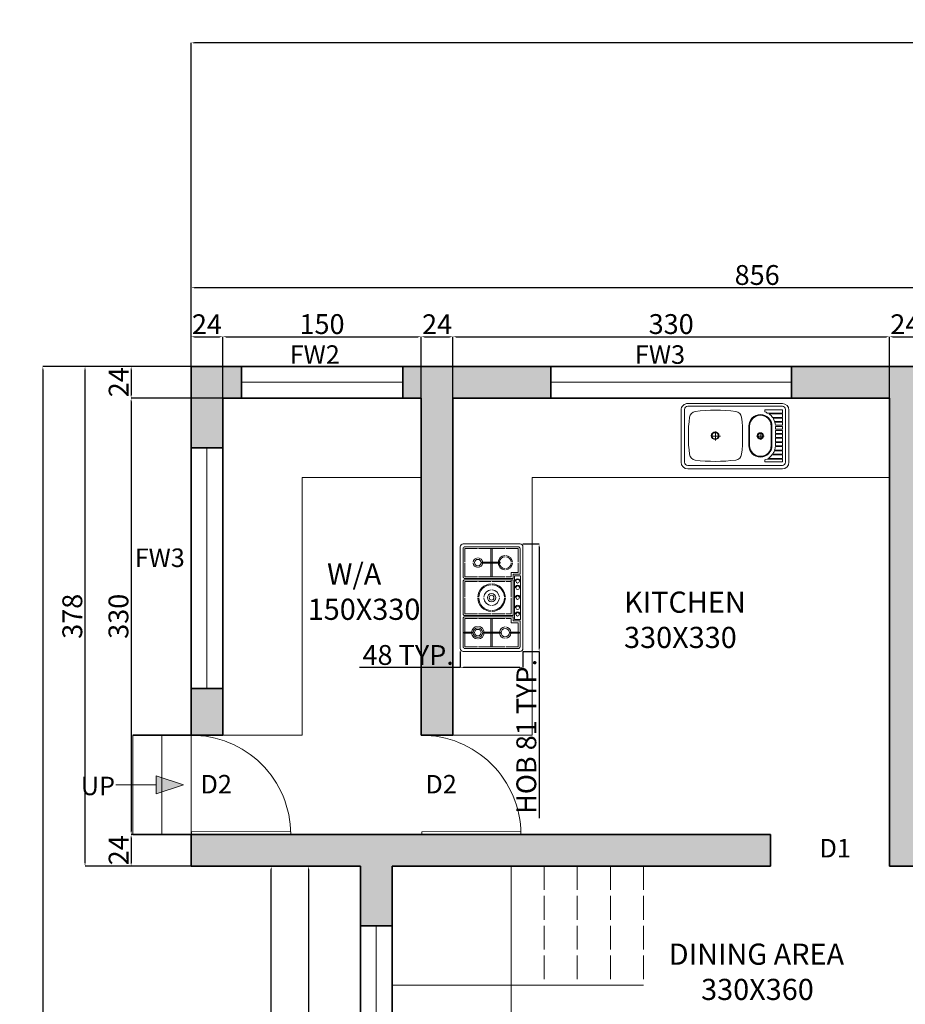
# Model space of a CAD drawing. Units: centimetres. Extents: x 2449 to 7478, y 778 to 2486.
# Tile 3 of 9: x 2449 to 3118, y 1732 to 2477. Entities that reach past the tile are written whole.
import ezdxf

# ---------------------------------------------------------------- set-up
doc = ezdxf.new("R2010")
doc.units = ezdxf.units.CM
doc.linetypes.add('ACAD_ISO02W100', pattern=[15, 12, -3])
for name, color, linetype, lineweight in [('A-ANNO-DIMS', 2, 'Continuous', 18), ('A-ANNO-SYMB', 8, 'Continuous', 18), ('A-ANNO-TEXT', 7, 'Continuous', 18), ('A-AREA-IDEN', 7, 'Continuous', 18), ('A-DOOR', 4, 'Continuous', 18), ('A-EQPM', 8, 'Continuous', 18), ('A-FLOR-CASE', 8, 'Continuous', 18), ('A-FLOR-FIXT', 8, 'Continuous', 18), ('A-FLOR-STRS', 7, 'Continuous', 18), ('A-FLOR-STRS-OVHD', 7, 'ACAD_ISO02W100', 13), ('A-WALL', 7, 'Continuous', 35), ('A-WALL-PATT', 7, 'Continuous', 13), ('Win', 1, 'Continuous', 18)]:
    doc.layers.add(name, color=color, linetype=linetype, lineweight=lineweight)
doc.styles.get("Standard").update_dxf_attribs({"font": 'arial.ttf'})
doc.dimstyles.new('ISO-25', dxfattribs={"dimtxt": 15, "dimasz": 2.5, "dimexe": 0, "dimexo": 0, "dimgap": 0, "dimtad": 1, "dimtxsty": 'Standard', "dimcen": 2.5, "dimadec": 0, "dimazin": 0, "dimtfac": 1, "dimtmove": 0, "dimatfit": 3, "dimfxl": 1, "dimarcsym": 0})

# ---------------------------------------------------------------- blocks, each defined once
blk = doc.blocks.new('sink 1')
for points in [[(-7.34, 1.48), (-7.34, 22.73)], [(-6.56, 1.48), (-6.56, 22.73)], [(5.86, 24.22), (-5.86, 24.22)], [(6.01, 23.43), (-5.86, 23.43)], [(6.72, 1.48), (6.72, 22.73)], [(7.34, 1.48), (7.34, 22.73)], [(1.09, 16.48), (-0.94, 16.48)], [(0, 15.39), (0, 17.42)], [(-2.09, 8.99), (2.28, 8.99)], [(-2.09, 8.84), (2.28, 8.84)], [(0, 5.55), (0, 7.26)], [(-5.78, 5.39), (-5.78, 5.39)], [(-5.31, 5.39), (-5.31, 5.39)], [(-5.16, 4.92), (-5.16, 4.92)], [(-5, 1.48), (-5, 4.69)], [(-4.84, 4.45), (-4.84, 4.45)], [(0.78, 6.33), (-0.78, 6.33)], [(5, 4.45), (5, 4.45)], [(5.16, 4.92), (5.16, 4.92)], [(5.94, 5.39), (5.94, 5.39)], [(-5, 1.48), (-4.22, 1.48), (-4.22, 3.83)], [(-4.22, 3.83), (-4.22, 3.83)], [(-4.06, 1.48), (-4.06, 3.69)], [(-4.06, 1.48), (-3.28, 1.48), (-3.28, 3.27)], [(-3.91, 3.52), (-3.91, 3.52)], [(-3.28, 3.2), (-3.28, 3.2)], [(-3.12, 3.2), (-3.12, 3.2)], [(-2.34, 3.05), (-2.34, 3.05)], [(-2.19, 3.05), (-2.19, 3.05)], [(-2.09, 3.99), (2.28, 3.99)], [(-2.09, 3.84), (2.28, 3.84)], [(-1.41, 3.05), (-1.41, 3.05)], [(-1.25, 3.05), (-1.25, 3.05)], [(-0.47, 1.48), (-1.25, 1.48), (-1.25, 3.05), (-0.47, 3.05)], [(-0.62, 3.05), (-0.62, 3.05)], [(-0.47, 1.48), (-0.47, 3.05)], [(-0.31, 3.05), (-0.31, 3.05)], [(0.47, 1.48), (-0.31, 1.48), (-0.31, 3.05), (0.47, 3.05)], [(0.31, 3.05), (0.31, 3.05)], [(0.47, 1.48), (0.47, 3.05)], [(0.62, 3.05), (0.62, 3.05)], [(1.25, 3.05), (1.25, 3.05)], [(1.56, 3.05), (1.56, 3.05)], [(2.19, 3.05), (2.19, 3.05)], [(2.5, 3.05), (2.5, 3.05)], [(3.12, 3.2), (3.12, 3.2)], [(3.28, 1.48), (4.06, 1.48), (4.06, 3.57)], [(3.28, 1.48), (3.28, 3.2)], [(3.44, 3.2), (3.44, 3.2)], [(4.06, 3.52), (4.06, 3.52)], [(4.22, 1.48), (4.22, 3.67)], [(4.37, 3.83), (4.37, 3.83)], [(6.01, 0.78), (-5.86, 0.78)], [(5.86, 0), (-5.86, 0)], [(-5.78, 1.48), (-5.78, 1.48)], [(-5.16, 1.48), (-5.16, 1.48)], [(-4.84, 1.48), (-4.84, 1.48)], [(-4.22, 1.48), (-4.22, 1.48)], [(-3.91, 1.48), (-3.91, 1.48)], [(-3.28, 1.48), (-3.28, 1.48)], [(-3.12, 1.48), (-3.12, 1.48)], [(-2.34, 1.48), (-2.34, 1.48)], [(-2.19, 1.48), (-2.19, 1.48)], [(-1.41, 1.48), (-1.41, 1.48)], [(-1.25, 1.48), (-1.25, 1.48)], [(-0.62, 1.48), (-0.62, 1.48)], [(-0.31, 1.48), (-0.31, 1.48)], [(0.31, 1.48), (0.31, 1.48)], [(0.62, 1.48), (0.62, 1.48)], [(1.25, 1.48), (1.25, 1.48)], [(1.56, 1.48), (1.56, 1.48)], [(2.19, 1.48), (2.19, 1.48)], [(2.5, 1.48), (2.5, 1.48)], [(3.12, 1.48), (3.12, 1.48)], [(3.44, 1.48), (3.44, 1.48)], [(4.06, 1.48), (4.06, 1.48)], [(4.37, 1.48), (4.37, 1.48)], [(5, 1.48), (5, 1.48)], [(5.16, 1.48), (5.16, 1.48)], [(5.94, 1.48), (5.94, 1.48)]]:
    blk.add_lwpolyline(points)
for points in [[(-5.16, 4.92), (-5.16, 1.48), (-5.78, 1.48), (-5.78, 5.39), (-5.31, 5.39, -0.068511), (-5.16, 4.92)], [(4.22, 1.48), (5, 1.48), (5, 4.45, -0.083542), (4.22, 3.67, -0.083542)], [(5.16, 4.92, 0.248301), (5.47, 5.39), (5.94, 5.39), (5.94, 1.48), (5.16, 1.48), (5.16, 4.92)], [(4.06, 3.57, -0.061679), (3.32, 3.22)]]:
    blk.add_lwpolyline(points, format="xyb")
for points in [[(-3.12, 3.22), (-3.12, 1.48), (-2.34, 1.48), (-2.34, 3.05, -0.06228)], [(2.5, 3.05), (2.5, 1.48), (3.12, 1.48), (3.12, 3.2, -0.050256)]]:
    blk.add_lwpolyline(points, format="xyb", close=True)
for points in [[(-2.19, 3.05), (-1.41, 3.05), (-1.41, 1.48), (-2.19, 1.48)], [(0.62, 3.05), (1.25, 3.05), (1.25, 1.48), (0.62, 1.48)], [(2.19, 1.48), (2.19, 3.05), (1.56, 3.05), (1.56, 1.48)]]:
    blk.add_lwpolyline(points, close=True)
for centre, radius in [((0.09, 16.57), 0.859), ((0.09, 16.57), 0.703), ((0.09, 6.41), 0.703), ((0.09, 6.41), 0.547)]:
    blk.add_circle(centre, radius)
for centre, radius, start, end in [((-5.86, 22.73), 1.48, 90, 180), ((-5.86, 22.73), 0.703, 90, 180), ((-3.87, 20.82), 1.53, 97.3256, 171.1849), ((0.09, -12.65), 35.23, 83.2159, 96.7841), ((4.06, 20.82), 1.53, 8.8151, 82.6744), ((5.86, 22.73), 1.48, 360, 90), ((6.01, 22.73), 0.703, 0, 90), ((30.19, 16.56), 35.85, 172.7947, 187.4213), ((-30, 16.56), 35.85, 352.5787, 7.2053), ((-3.89, 12.12), 1.48, 187.4212, 263.2159), ((4.08, 12.12), 1.48, 276.7841, 352.5788), ((-2.1, 6.41), 2.58, 90, 270), ((0.09, 45.63), 35.23, 263.2159, 276.7841), ((2.28, 6.41), 2.58, 270, 90), ((-2.1, 6.41), 2.42, 90, 270), ((2.28, 6.41), 2.42, 270, 90), ((-2.15, 6.48), 3.36, 212.1095, 232.0862), ((-2.1, 6.41), 3.36, 234.156, 249.3275), ((2.14, 6.36), 3.36, 289.8633, 290.5971), ((-5.86, 1.48), 1.48, 180, 270), ((-5.86, 1.48), 0.703, 180, 270), ((5.86, 1.48), 1.48, 270, 0), ((6.01, 1.48), 0.703, 270, 360)]:
    blk.add_arc(centre, radius, start, end)
blk = doc.blocks.new('STOVE')
for p, q in [((11.85, 19.7), (11.55, 19.7)), ((11.55, 16.92), (11.55, 19.7)), ((11.85, 16.92), (11.55, 16.92)), ((11.85, 16.92), (11.85, 19.7)), ((-11.85, 13.73), (-11.85, 7.62)), ((-11.85, 13.73), (-11.55, 13.73)), ((-11.55, 13.73), (-11.55, 7.62)), ((11.85, 13.23), (11.55, 13.23)), ((11.55, 13.23), (11.55, 7.57)), ((11.85, 13.23), (11.85, 7.57)), ((-11.85, 10.75), (-16.4, 10.75)), ((-11.85, 10.25), (-16.4, 10.25)), ((-7, 10.75), (-11.55, 10.75)), ((-7, 10.25), (-11.55, 10.25)), ((7, 10.75), (11.55, 10.75)), ((7, 10.25), (11.55, 10.25)), ((11.85, 10.75), (16.4, 10.75)), ((11.85, 10.25), (16.4, 10.25)), ((-11.85, 7.62), (-11.55, 7.62)), ((11.85, 7.57), (11.55, 7.57)), ((-7, 3.9), (-8.4, 3.9)), ((-7.8, 3.3), (-7.8, 1)), ((-6.4, 3.3), (-7.8, 3.3)), ((-5.4, 3.9), (-6, 3.9)), ((-5.4, 3.9), (-0.15, 3.9)), ((0.15, 3.9), (5.4, 3.9)), ((6.4, 3.3), (7.8, 3.3)), ((7, 3.9), (8.4, 3.9)), ((7.8, 3.3), (7.8, 1)), ((8.4, 3.9), (8.4, 1.6)), ((11.85, 4.28), (11.55, 4.28)), ((11.55, 4.28), (11.55, 1.3)), ((11.85, 4.28), (11.85, 1.3)), ((7.3, 2.8), (-7.3, 2.8)), ((-7.3, 2.8), (-7.3, 0.8)), ((7.3, 0.8), (-7.3, 0.8)), ((7.3, 2.8), (7.3, 0.8)), ((11.85, 1.3), (11.55, 1.3))]:
    blk.add_line(p, q)
for points in [[(-17, 21), (17, 21, -0.414214), (18, 20), (18, 1, -0.414214), (17, 0), (-17, 0, -0.414214), (-18, 1), (-18, 20, -0.414214)], [(6, 3.3), (-6, 3.3), (-6, 19.4, -0.414214), (-5.4, 20), (5.4, 20, -0.414214), (6, 19.4)]]:
    blk.add_lwpolyline(points, format="xyb", close=True)
for points in [[(-7.8, 1), (-16.4, 1, -0.414214), (-17, 1.6), (-17, 19.4, -0.414214), (-16.4, 20), (-7, 20, -0.414214), (-6.4, 19.4), (-6.4, 3.3)], [(6.4, 19.4, -0.414214), (7, 20), (16.4, 20, -0.414214), (17, 19.4), (17, 1.6, -0.414214), (16.4, 1), (7.8, 1)]]:
    blk.add_lwpolyline(points, format="xyb")
for points in [[(-16.4, 15.22), (-16.4, 19.4), (-11.85, 19.4)], [(-11.55, 19.4), (-7, 19.4), (-7, 15.22)], [(-5.4, 15.22), (-5.4, 19.4), (-0.15, 19.4)], [(0.15, 19.4), (5.4, 19.4), (5.4, 15.22)], [(6.4, 3.3), (6.4, 19.4)], [(7, 15.22), (7, 19.4), (11.55, 19.4)], [(11.85, 19.4), (16.4, 19.4), (16.4, 15.22)], [(-16.4, 6.08), (-16.4, 14.92)], [(-7, 14.92), (-7, 6.08)], [(-5.4, 10.65), (-5.4, 14.92)], [(5.4, 14.92), (5.4, 10.65)], [(7, 6.08), (7, 14.92)], [(16.4, 14.92), (16.4, 6.08)], [(-5.4, 6.08), (-5.4, 10.35)], [(5.4, 10.35), (5.4, 6.08)], [(-11.85, 1.6), (-16.4, 1.6), (-16.4, 5.77)], [(-8.4, 3.9), (-8.4, 1.6), (-11.55, 1.6)], [(-7, 5.77), (-7, 3.9)], [(-5.4, 3.9), (-5.4, 5.77)], [(5.4, 5.77), (5.4, 3.9)], [(7, 3.9), (7, 5.77)], [(16.4, 5.77), (16.4, 1.6), (11.85, 1.6)], [(11.55, 1.6), (8.4, 1.6)]]:
    blk.add_lwpolyline(points)
for centre, radius in [((11.7, 15.07), 1.6), ((-11.7, 15.07), 1.1), ((11.7, 15.07), 1.1), ((0, 10.5), 1.4), ((0, 10.5), 0.8), ((11.7, 5.93), 1.4), ((-5.49, 1.8), 0.6), ((-3.3, 1.8), 0.6), ((0, 1.8), 0.6), ((3.39, 1.8), 0.6), ((5.57, 1.8), 0.6)]:
    blk.add_circle(centre, radius)
for centre, radius, start, end in [((-11.7, 15.07), 1.6, 95.3794, 174.6206), ((-11.7, 15.07), 1.6, 5.3794, 84.6206), ((11.7, 15.07), 2.1, 94.096, 175.904), ((11.7, 15.07), 2.1, 4.096, 85.904), ((-11.7, 15.07), 1.6, 185.3794, 264.6206), ((-11.7, 15.07), 1.6, 275.3794, 354.6206), ((0, 10.5), 4.6, 91.8687, 178.1313), ((0, 10.5), 4.3, 91.9991, 178.0009), ((0, 10.5), 4.6, 1.8687, 88.1313), ((0, 10.5), 4.3, 1.9991, 88.0009), ((11.7, 15.07), 2.1, 184.096, 265.904), ((11.7, 15.07), 2.1, 274.096, 355.904), ((0, 10.5), 4.6, 181.8687, 268.1313), ((0, 10.5), 4.3, 181.9991, 268.0009), ((0, 10.5), 2.6, 93.3074, 176.6926), ((0, 10.5), 2.6, 183.3074, 266.6926), ((0, 10.5), 2.6, 3.3074, 86.6926), ((0, 10.5), 4.6, 271.8687, 358.1313), ((0, 10.5), 4.3, 271.9991, 358.0009), ((0, 10.5), 2.6, 273.3074, 356.6926), ((-11.7, 5.93), 2.4, 93.5833, 176.4167), ((-11.7, 5.93), 2, 94.3012, 175.6988), ((-11.7, 5.93), 2.4, 3.5833, 86.4167), ((-11.7, 5.93), 2, 4.3012, 85.6988), ((11.7, 5.93), 1.9, 94.5281, 175.4719), ((11.7, 5.93), 1.9, 4.5281, 85.4719), ((-11.7, 5.93), 2.4, 183.5833, 266.4167), ((-11.7, 5.93), 2, 184.3012, 265.6988), ((-11.7, 5.93), 2.4, 273.5833, 356.4167), ((-11.7, 5.93), 2, 274.3012, 355.6988), ((11.7, 5.93), 1.9, 184.5281, 265.4719), ((11.7, 5.93), 1.9, 274.5281, 355.4719), ((-5.49, 1.8), 0.846, 89.9979, 270), ((-3.3, 1.8), 0.846, 89.9979, 270), ((0, 1.8), 0.846, 89.9979, 270), ((3.39, 1.8), 0.846, 89.9979, 270), ((5.57, 1.8), 0.846, 89.9979, 270)]:
    blk.add_arc(centre, radius, start, end)
blk = doc.blocks.new('*D15')
at = {"layer": 'A-ANNO-DIMS', "color": 0, "lineweight": -2, "transparency": 16777216}
for p, q in [((2578.09, 2214.34), (2578.09, 2236.78)), ((2580.59, 2236.78), (2599.59, 2236.78)), ((2602.09, 2190.34), (2602.09, 2236.78))]:
    blk.add_line(p, q, dxfattribs=at)
at = {"layer": 'A-ANNO-DIMS', "color": 0, "transparency": 16777216}
for points in [[(2580.59, 2237.19), (2580.59, 2236.36), (2578.09, 2236.78)], [(2599.59, 2237.19), (2599.59, 2236.36), (2602.09, 2236.78)]]:
    blk.add_solid(points, dxfattribs=at)
at = {"layer": 'Defpoints', "color": 0, "transparency": 16777216}
for p in [(2602.09, 2236.78), (2578.09, 2214.34), (2602.09, 2190.34)]:
    blk.add_point(p, dxfattribs=at)
at = {"layer": 'A-ANNO-DIMS', "color": 0, "transparency": 16777216, "insert": (2590.09, 2244.31), "char_height": 15, "attachment_point": 5}
blk.add_mtext('24', dxfattribs=at)
blk = doc.blocks.new('*D16')
at = {"layer": 'A-ANNO-DIMS', "color": 0, "lineweight": -2, "transparency": 16777216}
for p, q in [((2602.09, 2190.34), (2602.09, 2236.78)), ((2604.59, 2236.78), (2749.59, 2236.78)), ((2752.09, 2190.34), (2752.09, 2236.78))]:
    blk.add_line(p, q, dxfattribs=at)
at = {"layer": 'A-ANNO-DIMS', "color": 0, "transparency": 16777216}
for points in [[(2604.59, 2237.19), (2604.59, 2236.36), (2602.09, 2236.78)], [(2749.59, 2237.19), (2749.59, 2236.36), (2752.09, 2236.78)]]:
    blk.add_solid(points, dxfattribs=at)
at = {"layer": 'Defpoints', "color": 0, "transparency": 16777216}
for p in [(2752.09, 2236.78), (2602.09, 2190.34), (2752.09, 2190.34)]:
    blk.add_point(p, dxfattribs=at)
at = {"layer": 'A-ANNO-DIMS', "color": 0, "transparency": 16777216, "insert": (2677.09, 2244.43), "char_height": 15, "attachment_point": 5}
blk.add_mtext('150', dxfattribs=at)
blk = doc.blocks.new('*D17')
at = {"layer": 'A-ANNO-DIMS', "color": 0, "lineweight": -2, "transparency": 16777216}
for p, q in [((2752.09, 2190.34), (2752.09, 2236.78)), ((2754.59, 2236.78), (2773.59, 2236.78)), ((2776.09, 2190.34), (2776.09, 2236.78))]:
    blk.add_line(p, q, dxfattribs=at)
at = {"layer": 'A-ANNO-DIMS', "color": 0, "transparency": 16777216}
for points in [[(2754.59, 2237.19), (2754.59, 2236.36), (2752.09, 2236.78)], [(2773.59, 2237.19), (2773.59, 2236.36), (2776.09, 2236.78)]]:
    blk.add_solid(points, dxfattribs=at)
at = {"layer": 'Defpoints', "color": 0, "transparency": 16777216}
for p in [(2776.09, 2236.78), (2752.09, 2190.34), (2776.09, 2190.34)]:
    blk.add_point(p, dxfattribs=at)
at = {"layer": 'A-ANNO-DIMS', "color": 0, "transparency": 16777216, "insert": (2764.09, 2244.31), "char_height": 15, "attachment_point": 5}
blk.add_mtext('24', dxfattribs=at)
blk = doc.blocks.new('*D18')
at = {"layer": 'A-ANNO-DIMS', "color": 0, "lineweight": -2, "transparency": 16777216}
for p, q in [((2776.09, 2190.34), (2776.09, 2236.78)), ((2778.59, 2236.78), (3103.59, 2236.78)), ((3106.09, 2190.34), (3106.09, 2236.78))]:
    blk.add_line(p, q, dxfattribs=at)
at = {"layer": 'A-ANNO-DIMS', "color": 0, "transparency": 16777216}
for points in [[(2778.59, 2237.19), (2778.59, 2236.36), (2776.09, 2236.78)], [(3103.59, 2237.19), (3103.59, 2236.36), (3106.09, 2236.78)]]:
    blk.add_solid(points, dxfattribs=at)
at = {"layer": 'Defpoints', "color": 0, "transparency": 16777216}
for p in [(3106.09, 2236.78), (2776.09, 2190.34), (3106.09, 2190.34)]:
    blk.add_point(p, dxfattribs=at)
at = {"layer": 'A-ANNO-DIMS', "color": 0, "transparency": 16777216, "insert": (2941.09, 2244.44), "char_height": 15, "attachment_point": 5}
blk.add_mtext('330', dxfattribs=at)
blk = doc.blocks.new('*D19')
at = {"layer": 'A-ANNO-DIMS', "color": 0, "lineweight": -2, "transparency": 16777216}
for p, q in [((3106.09, 2190.34), (3106.09, 2236.78)), ((3108.59, 2236.78), (3127.59, 2236.78)), ((3130.09, 2190.34), (3130.09, 2236.78))]:
    blk.add_line(p, q, dxfattribs=at)
at = {"layer": 'A-ANNO-DIMS', "color": 0, "transparency": 16777216}
for points in [[(3108.59, 2237.19), (3108.59, 2236.36), (3106.09, 2236.78)], [(3127.59, 2237.19), (3127.59, 2236.36), (3130.09, 2236.78)]]:
    blk.add_solid(points, dxfattribs=at)
at = {"layer": 'Defpoints', "color": 0, "transparency": 16777216}
for p in [(3130.09, 2236.78), (3106.09, 2190.34), (3130.09, 2190.34)]:
    blk.add_point(p, dxfattribs=at)
at = {"layer": 'A-ANNO-DIMS', "color": 0, "transparency": 16777216, "insert": (3118.09, 2244.31), "char_height": 15, "attachment_point": 5}
blk.add_mtext('24', dxfattribs=at)
blk = doc.blocks.new('*D26')
at = {"layer": 'A-ANNO-DIMS', "color": 0, "lineweight": -2, "transparency": 16777216}
for p, q in [((2578.09, 2214.34), (2578.09, 2273.89)), ((3431.59, 2273.89), (2580.59, 2273.89)), ((3434.09, 2214.34), (3434.09, 2273.89))]:
    blk.add_line(p, q, dxfattribs=at)
at = {"layer": 'A-ANNO-DIMS', "color": 0, "transparency": 16777216}
for points in [[(2580.59, 2274.31), (2580.59, 2273.47), (2578.09, 2273.89)], [(3431.59, 2274.31), (3431.59, 2273.47), (3434.09, 2273.89)]]:
    blk.add_solid(points, dxfattribs=at)
at = {"layer": 'Defpoints', "color": 0, "transparency": 16777216}
for p in [(2578.09, 2273.89), (2578.09, 2214.34), (3434.09, 2214.34)]:
    blk.add_point(p, dxfattribs=at)
at = {"layer": 'A-ANNO-DIMS', "color": 0, "transparency": 16777216, "insert": (3006.09, 2281.55), "char_height": 15, "attachment_point": 5}
blk.add_mtext('856', dxfattribs=at)
blk = doc.blocks.new('*D28')
at = {"layer": 'A-ANNO-DIMS', "color": 0, "lineweight": -2, "transparency": 16777216}
for p, q in [((2578.09, 2214.34), (2578.09, 2459.09)), ((3809.59, 2459.09), (2580.59, 2459.09)), ((3812.09, 2382.34), (3812.09, 2459.09))]:
    blk.add_line(p, q, dxfattribs=at)
at = {"layer": 'A-ANNO-DIMS', "color": 0, "transparency": 16777216}
for points in [[(2580.59, 2459.51), (2580.59, 2458.68), (2578.09, 2459.09)], [(3809.59, 2459.51), (3809.59, 2458.68), (3812.09, 2459.09)]]:
    blk.add_solid(points, dxfattribs=at)
at = {"layer": 'Defpoints', "color": 0, "transparency": 16777216}
for p in [(2578.09, 2459.09), (3812.09, 2382.34), (2578.09, 2214.34)]:
    blk.add_point(p, dxfattribs=at)
at = {"layer": 'A-ANNO-DIMS', "color": 0, "transparency": 16777216, "insert": (3195.09, 2466.76), "char_height": 15, "attachment_point": 5}
blk.add_mtext('1234', dxfattribs=at)
blk = doc.blocks.new('*D29')
at = {"layer": 'A-ANNO-DIMS', "color": 0, "lineweight": -2, "transparency": 16777216}
for p, q in [((2578.09, 2214.34), (2532.79, 2214.34)), ((2532.79, 2211.84), (2532.79, 2192.84)), ((2602.09, 2190.34), (2532.79, 2190.34))]:
    blk.add_line(p, q, dxfattribs=at)
at = {"layer": 'A-ANNO-DIMS', "color": 0, "transparency": 16777216}
for points in [[(2532.37, 2211.84), (2533.2, 2211.84), (2532.79, 2214.34)], [(2532.37, 2192.84), (2533.2, 2192.84), (2532.79, 2190.34)]]:
    blk.add_solid(points, dxfattribs=at)
at = {"layer": 'Defpoints', "color": 0, "transparency": 16777216}
for p in [(2578.09, 2214.34), (2532.79, 2190.34), (2602.09, 2190.34)]:
    blk.add_point(p, dxfattribs=at)
at = {"layer": 'A-ANNO-DIMS', "color": 0, "transparency": 16777216, "insert": (2525.26, 2202.34), "char_height": 15, "attachment_point": 5, "rotation": 90}
blk.add_mtext('24', dxfattribs=at)
blk = doc.blocks.new('*D30')
at = {"layer": 'A-ANNO-DIMS', "color": 0, "lineweight": -2, "transparency": 16777216}
for p, q in [((2602.09, 2190.34), (2532.79, 2190.34)), ((2532.79, 2187.84), (2532.79, 1862.84)), ((2578.09, 1860.34), (2532.79, 1860.34))]:
    blk.add_line(p, q, dxfattribs=at)
at = {"layer": 'A-ANNO-DIMS', "color": 0, "transparency": 16777216}
for points in [[(2532.37, 2187.84), (2533.2, 2187.84), (2532.79, 2190.34)], [(2532.37, 1862.84), (2533.2, 1862.84), (2532.79, 1860.34)]]:
    blk.add_solid(points, dxfattribs=at)
at = {"layer": 'Defpoints', "color": 0, "transparency": 16777216}
for p in [(2602.09, 2190.34), (2532.79, 1860.34), (2578.09, 1860.34)]:
    blk.add_point(p, dxfattribs=at)
at = {"layer": 'A-ANNO-DIMS', "color": 0, "transparency": 16777216, "insert": (2525.12, 2025.34), "char_height": 15, "attachment_point": 5, "rotation": 90}
blk.add_mtext('330', dxfattribs=at)
blk = doc.blocks.new('*D31')
at = {"layer": 'A-ANNO-DIMS', "color": 0, "lineweight": -2, "transparency": 16777216}
for p, q in [((2578.09, 1860.34), (2532.79, 1860.34)), ((2532.79, 1857.84), (2532.79, 1838.84)), ((2578.09, 1836.34), (2532.79, 1836.34))]:
    blk.add_line(p, q, dxfattribs=at)
at = {"layer": 'A-ANNO-DIMS', "color": 0, "transparency": 16777216}
for points in [[(2532.37, 1857.84), (2533.2, 1857.84), (2532.79, 1860.34)], [(2532.37, 1838.84), (2533.2, 1838.84), (2532.79, 1836.34)]]:
    blk.add_solid(points, dxfattribs=at)
at = {"layer": 'Defpoints', "color": 0, "transparency": 16777216}
for p in [(2578.09, 1860.34), (2532.79, 1836.34), (2578.09, 1836.34)]:
    blk.add_point(p, dxfattribs=at)
at = {"layer": 'A-ANNO-DIMS', "color": 0, "transparency": 16777216, "insert": (2525.26, 1848.34), "char_height": 15, "attachment_point": 5, "rotation": 90}
blk.add_mtext('24', dxfattribs=at)
blk = doc.blocks.new('*D32')
at = {"layer": 'A-ANNO-DIMS', "color": 0, "lineweight": -2, "transparency": 16777216}
for p, q in [((2706.09, 1836.34), (2666.8, 1836.34)), ((2666.8, 1833.84), (2666.8, 1478.84)), ((2730.09, 1476.34), (2666.8, 1476.34))]:
    blk.add_line(p, q, dxfattribs=at)
at = {"layer": 'A-ANNO-DIMS', "color": 0, "transparency": 16777216}
for points in [[(2666.38, 1833.84), (2667.22, 1833.84), (2666.8, 1836.34)], [(2666.38, 1478.84), (2667.22, 1478.84), (2666.8, 1476.34)]]:
    blk.add_solid(points, dxfattribs=at)
at = {"layer": 'Defpoints', "color": 0, "transparency": 16777216}
for p in [(2706.09, 1836.34), (2666.8, 1476.34), (2730.09, 1476.34)]:
    blk.add_point(p, dxfattribs=at)
at = {"layer": 'A-ANNO-DIMS', "color": 0, "transparency": 16777216, "insert": (2659.14, 1656.34), "char_height": 15, "attachment_point": 5, "rotation": 90}
blk.add_mtext('360', dxfattribs=at)
blk = doc.blocks.new('*D36')
at = {"layer": 'A-ANNO-DIMS', "color": 0, "lineweight": -2, "transparency": 16777216}
for p, q in [((2706.09, 1836.34), (2638.68, 1836.34)), ((2638.68, 1070.84), (2638.68, 1833.84)), ((2706.09, 1068.34), (2638.68, 1068.34))]:
    blk.add_line(p, q, dxfattribs=at)
at = {"layer": 'A-ANNO-DIMS', "color": 0, "transparency": 16777216}
for points in [[(2638.26, 1833.84), (2639.09, 1833.84), (2638.68, 1836.34)], [(2638.26, 1070.84), (2639.09, 1070.84), (2638.68, 1068.34)]]:
    blk.add_solid(points, dxfattribs=at)
at = {"layer": 'Defpoints', "color": 0, "transparency": 16777216}
for p in [(2638.68, 1836.34), (2706.09, 1836.34), (2706.09, 1068.34)]:
    blk.add_point(p, dxfattribs=at)
at = {"layer": 'A-ANNO-DIMS', "color": 0, "transparency": 16777216, "insert": (2631.02, 1452.34), "char_height": 15, "attachment_point": 5, "rotation": 90}
blk.add_mtext('768', dxfattribs=at)
blk = doc.blocks.new('*D37')
at = {"layer": 'A-ANNO-DIMS', "color": 0, "lineweight": -2, "transparency": 16777216}
for p, q in [((2578.09, 2214.34), (2497.9, 2214.34)), ((2497.9, 1838.84), (2497.9, 2211.84)), ((2578.09, 1836.34), (2497.9, 1836.34))]:
    blk.add_line(p, q, dxfattribs=at)
at = {"layer": 'A-ANNO-DIMS', "color": 0, "transparency": 16777216}
for points in [[(2497.49, 2211.84), (2498.32, 2211.84), (2497.9, 2214.34)], [(2497.49, 1838.84), (2498.32, 1838.84), (2497.9, 1836.34)]]:
    blk.add_solid(points, dxfattribs=at)
at = {"layer": 'Defpoints', "color": 0, "transparency": 16777216}
for p in [(2497.9, 2214.34), (2578.09, 2214.34), (2578.09, 1836.34)]:
    blk.add_point(p, dxfattribs=at)
at = {"layer": 'A-ANNO-DIMS', "color": 0, "transparency": 16777216, "insert": (2490.24, 2025.34), "char_height": 15, "attachment_point": 5, "rotation": 90}
blk.add_mtext('378', dxfattribs=at)
blk = doc.blocks.new('*D38')
at = {"layer": 'A-ANNO-DIMS', "color": 0, "lineweight": -2, "transparency": 16777216}
for p, q in [((2578.09, 2214.34), (2466.02, 2214.34)), ((2466.02, 2211.84), (2466.02, 1070.84)), ((2706.09, 1068.34), (2466.02, 1068.34))]:
    blk.add_line(p, q, dxfattribs=at)
at = {"layer": 'A-ANNO-DIMS', "color": 0, "transparency": 16777216}
for points in [[(2465.6, 2211.84), (2466.43, 2211.84), (2466.02, 2214.34)], [(2465.6, 1070.84), (2466.43, 1070.84), (2466.02, 1068.34)]]:
    blk.add_solid(points, dxfattribs=at)
at = {"layer": 'Defpoints', "color": 0, "transparency": 16777216}
for p in [(2578.09, 2214.34), (2466.02, 1068.34), (2706.09, 1068.34)]:
    blk.add_point(p, dxfattribs=at)
at = {"layer": 'A-ANNO-DIMS', "color": 0, "transparency": 16777216, "insert": (2458.36, 1641.34), "char_height": 15, "attachment_point": 5, "rotation": 90}
blk.add_mtext('1146', dxfattribs=at)
blk = doc.blocks.new('3')
for p, q in [((5936.31, 1821.57), (5936.31, 1746.57)), ((5938.31, 1821.57), (5938.31, 1746.57)), ((5938.31, 1746.57), (5936.31, 1746.57))]:
    blk.add_line(p, q)
blk.add_arc((5936.31, 1746.57), 75, 0, 90)
blk = doc.blocks.new('COUNTER-KITCHEN')
for p, q in [((0, 0), (270, 0)), ((0, 0), (0, -195)), ((0, -195), (-60, -195))]:
    blk.add_line(p, q)
blk = doc.blocks.new('COUNTER-UTILITY')
for p, q in [((0, 0), (90, 0)), ((0, 0), (0, -195)), ((-60, -195), (0, -195))]:
    blk.add_line(p, q)
blk = doc.blocks.new('ARROW-ENTRY-UP')
at = {"transparency": 33554687}
h = blk.add_hatch(color=256, dxfattribs=at)
h.dxf.hatch_style = 1
h.paths.add_polyline_path([(-6.84, 30.34), (6.84, 30.34), (0, 51.25)])
blk.add_line((0, 30.34), (0, 0))
blk.add_lwpolyline([(0, 51.25), (-6.84, 30.34), (6.84, 30.34)], close=True)
blk = doc.blocks.new('*D92')
at = {"layer": 'A-ANNO-DIMS', "color": 0, "lineweight": -2, "transparency": 16777216}
for p, q in [((2829.04, 2080.17), (2841.26, 2080.17)), ((2841.26, 2077.67), (2841.26, 2001.23)), ((2829.04, 1998.73), (2841.26, 1998.73)), ((2841.26, 1998.73), (2841.26, 1872.79))]:
    blk.add_line(p, q, dxfattribs=at)
at = {"layer": 'A-ANNO-DIMS', "color": 0, "transparency": 16777216}
for points in [[(2840.84, 2077.67), (2841.68, 2077.67), (2841.26, 2080.17)], [(2840.84, 2001.23), (2841.68, 2001.23), (2841.26, 1998.73)]]:
    blk.add_solid(points, dxfattribs=at)
at = {"layer": 'Defpoints', "color": 0, "transparency": 16777216}
for p in [(2829.04, 2080.17), (2829.04, 1998.73), (2841.26, 1998.73)]:
    blk.add_point(p, dxfattribs=at)
at = {"layer": 'A-ANNO-DIMS', "color": 0, "transparency": 16777216, "insert": (2833.5, 1934.51), "char_height": 15, "attachment_point": 5, "rotation": 90}
blk.add_mtext('HOB 81 TYP.', dxfattribs=at)
blk = doc.blocks.new('*D93')
at = {"layer": 'A-ANNO-DIMS', "color": 0, "lineweight": -2, "transparency": 16777216}
for p, q in [((2781.54, 1998.73), (2781.54, 1986.51)), ((2829.04, 1998.73), (2829.04, 1986.51)), ((2781.54, 1986.51), (2705.42, 1986.51)), ((2826.54, 1986.51), (2784.04, 1986.51))]:
    blk.add_line(p, q, dxfattribs=at)
at = {"layer": 'A-ANNO-DIMS', "color": 0, "transparency": 16777216}
for points in [[(2784.04, 1986.93), (2784.04, 1986.1), (2781.54, 1986.51)], [(2826.54, 1986.93), (2826.54, 1986.1), (2829.04, 1986.51)]]:
    blk.add_solid(points, dxfattribs=at)
at = {"layer": 'Defpoints', "color": 0, "transparency": 16777216}
for p in [(2781.54, 1998.73), (2829.04, 1998.73), (2781.54, 1986.51)]:
    blk.add_point(p, dxfattribs=at)
at = {"layer": 'A-ANNO-DIMS', "color": 0, "transparency": 16777216, "insert": (2742.23, 1994.17), "char_height": 15, "attachment_point": 5}
blk.add_mtext('48 TYP.', dxfattribs=at)

msp = doc.modelspace()

# ---------------------------------------------------------------- hatches: boundary and pattern name
at = {"layer": 'A-WALL-PATT'}
h = msp.add_hatch(color=256, dxfattribs=at)
h.dxf.hatch_style = 1
h.paths.add_polyline_path([(3060.088, 1092.34), (2986.088, 1092.34), (2986.088, 1068.34), (3084.088, 1068.34), (3084.088, 1476.34), (3060.088, 1476.34)])
h.paths.add_polyline_path([(2706.088, 1167.34), (2730.088, 1167.34), (2730.088, 1377.34), (2706.088, 1377.34)])
h.paths.add_polyline_path([(2804.088, 1068.34), (2804.088, 1092.34), (2730.088, 1092.34), (2730.088, 1112.34), (2706.088, 1112.34), (2706.088, 1068.34)])
h.paths.add_polyline_path([(2730.088, 1551.34), (2706.088, 1551.34), (2706.088, 1432.34), (2730.088, 1432.34), (2730.088, 1452.34), (2970.088, 1452.34), (2970.088, 1476.34), (2730.088, 1476.34)])
h.paths.add_polyline_path([(3434.088, 1654.34), (3434.088, 1266.34), (3405.088, 1266.34), (3405.088, 1242.34), (3458.088, 1242.34), (3458.088, 1404.34), (3482.088, 1404.34), (3482.088, 1428.34), (3458.088, 1428.34), (3458.088, 1678.34), (3260.088, 1678.34), (3260.088, 1654.34)])
h.paths.add_polyline_path([(3223.088, 1266.34), (3194.088, 1266.34), (3194.088, 1242.34), (3223.088, 1242.34)])
h.paths.add_polyline_path([(3812.088, 1506.339), (3788.088, 1506.339), (3788.088, 1428.34), (3764.088, 1428.34), (3764.088, 1404.34), (3812.088, 1404.34)])
h.paths.add_polyline_path([(3709.088, 1404.34), (3709.088, 1428.34), (3537.088, 1428.34), (3537.088, 1404.34)])
h.paths.add_polyline_path([(3788.088, 1688.339), (3812.088, 1688.339), (3812.088, 1826.34), (3788.088, 1826.34), (3788.088, 1792.34), (3647.088, 1792.34), (3647.088, 1768.34), (3788.088, 1768.34)])
h.paths.add_polyline_path([(3788.088, 1956.34), (3548.088, 1956.34), (3548.088, 1792.34), (3434.088, 1792.34), (3434.088, 1768.34), (3572.088, 1768.34), (3572.088, 1932.34), (3788.088, 1932.34), (3788.088, 1898.34), (3812.088, 1898.34), (3812.088, 2065.339), (3788.088, 2065.339)])
h.paths.add_polyline_path([(3788.088, 2358.34), (3788.088, 2247.339), (3812.088, 2247.339), (3812.088, 2382.34), (3764.088, 2382.34), (3764.088, 2358.34)])
h.paths.add_polyline_path([(3537.088, 2382.34), (3537.088, 2358.34), (3709.088, 2358.34), (3709.088, 2382.34)])
h.paths.add_polyline_path([(3458.088, 2358.34), (3482.088, 2358.34), (3482.088, 2382.34), (3434.088, 2382.34), (3434.088, 2214.34), (3395.088, 2214.34), (3395.088, 2190.34), (3434.088, 2190.34), (3434.088, 2065.34), (3458.088, 2065.34)])
h.paths.add_polyline_path([(3231.088, 2214.34), (3231.088, 2190.34), (3260.088, 2190.34), (3260.088, 1966.34), (3434.088, 1966.34), (3434.088, 1932.34), (3458.088, 1932.34), (3458.088, 1990.34), (3284.088, 1990.34), (3284.088, 2190.34), (3323.088, 2190.34), (3323.088, 2214.34)])
h.paths.add_polyline_path([(3130.088, 2190.34), (3159.088, 2190.34), (3159.088, 2214.34), (3032.088, 2214.34), (3032.088, 2190.34), (3106.088, 2190.34), (3106.088, 1836.34), (3130.088, 1836.34), (3130.088, 1966.34), (3185.088, 1966.34), (3185.088, 1990.34), (3130.088, 1990.34)])
h.paths.add_polyline_path([(2738.088, 2214.34), (2738.088, 2190.34), (2752.088, 2190.34), (2752.088, 1935.34), (2776.088, 1935.34), (2776.088, 2190.34), (2850.088, 2190.34), (2850.088, 2214.34)])
h.paths.add_polyline_path([(2578.088, 2152.839), (2602.088, 2152.839), (2602.088, 2190.34), (2616.088, 2190.34), (2616.088, 2214.34), (2578.088, 2214.34)])
h.paths.add_polyline_path([(2578.088, 1935.34), (2602.088, 1935.34), (2602.088, 1970.839), (2578.088, 1970.839)])
h.paths.add_polyline_path([(2706.088, 1836.34), (2706.088, 1791.34), (2730.088, 1791.34), (2730.088, 1836.34), (3016.088, 1836.34), (3016.088, 1860.34), (2578.088, 1860.34), (2578.088, 1836.34)])

# ---------------------------------------------------------------- linework, layer by layer
at = {"layer": 'A-FLOR-STRS'}
for p, q in [((2534.088, 1935.34), (2534.088, 1860.34)), ((2556.088, 1935.34), (2556.088, 1860.34)), ((2578.088, 1935.34), (2578.088, 1860.34)), ((2820.088, 1836.34), (2820.088, 1476.34)), ((2730.088, 1746.34), (2920.088, 1746.34))]:
    msp.add_line(p, q, dxfattribs=at)
at = {"layer": 'A-FLOR-STRS-OVHD', "ltscale": 1.5}
for p, q in [((2845.088, 1836.34), (2845.088, 1746.34)), ((2870.088, 1836.34), (2870.088, 1746.34)), ((2895.088, 1836.34), (2895.088, 1746.34)), ((2920.088, 1836.34), (2920.088, 1746.34))]:
    msp.add_line(p, q, dxfattribs=at)
at = {"layer": 'A-WALL'}
for p, q in [((2578.088, 2214.34), (3434.088, 2214.34)), ((2578.088, 2214.34), (2578.088, 1935.34)), ((2616.088, 2190.34), (2616.088, 2214.34)), ((2738.088, 2190.34), (2738.088, 2214.34)), ((2850.088, 2190.34), (2850.088, 2214.34)), ((3032.088, 2190.34), (3032.088, 2214.34)), ((2602.088, 2190.34), (2752.088, 2190.34)), ((2602.088, 2190.34), (2602.088, 1935.34)), ((2752.088, 2190.34), (2752.088, 1935.34)), ((2776.088, 2190.34), (2776.088, 1935.34)), ((2776.088, 2190.34), (3106.088, 2190.34)), ((3106.088, 2190.34), (3106.088, 1836.34)), ((2578.088, 2152.839), (2602.088, 2152.839)), ((2578.088, 1970.839), (2602.088, 1970.839)), ((2534.088, 1935.34), (2602.088, 1935.34)), ((2752.088, 1935.34), (2776.088, 1935.34)), ((2534.088, 1860.34), (3016.088, 1860.34)), ((2578.088, 1860.34), (2578.088, 1836.34)), ((3016.088, 1860.34), (3016.088, 1836.34)), ((2578.088, 1836.34), (2706.088, 1836.34)), ((2706.088, 1836.34), (2706.088, 1068.34)), ((2730.088, 1836.34), (2730.088, 1476.34)), ((2730.088, 1836.34), (3016.088, 1836.34)), ((3106.088, 1836.34), (3130.088, 1836.34)), ((2730.088, 1791.34), (2706.088, 1791.34))]:
    msp.add_line(p, q, dxfattribs=at)
at = {"layer": 'Win'}
for p, q in [((2616.088, 2202.34), (2738.088, 2202.34)), ((2850.088, 2202.34), (3032.088, 2202.34)), ((2590.088, 2152.839), (2590.088, 1970.839)), ((2718.088, 1791.34), (2718.088, 1551.34))]:
    msp.add_line(p, q, dxfattribs=at)

# ---------------------------------------------------------------- block references
at = {"layer": 'A-ANNO-SYMB', "rotation": 269.9999999999996}
msp.add_blockref('ARROW-ENTRY-UP', (2521.232, 1897.84), dxfattribs=at)
at = {"layer": 'A-DOOR', "xscale": -1, "rotation": 270.2708478329989}
for p in [(859.957, -4084.159), (1033.957, -4084.159)]:
    msp.add_blockref('3', p, dxfattribs=at)
at = {"layer": 'A-EQPM', "xscale": -2.262184600755962, "yscale": 2.262184600755962, "zscale": 2.262184600755962, "rotation": 90}
msp.add_blockref('STOVE', (2829.043, 2039.449), dxfattribs=at)
at = {"layer": 'A-FLOR-CASE'}
for name, p in [('COUNTER-UTILITY', (2662.088, 2130.34)), ('COUNTER-KITCHEN', (2836.088, 2130.34))]:
    msp.add_blockref(name, p, dxfattribs=at)
at = {"layer": 'A-FLOR-FIXT', "xscale": 3.367959604697591, "yscale": 3.367959604697591, "zscale": 3.367959604697591, "rotation": 90}
msp.add_blockref('sink 1', (3030.135, 2161.57), dxfattribs=at)

# ---------------------------------------------------------------- texts
at = {"layer": 'A-ANNO-TEXT', "char_height": 14, "attachment_point": 1}
for s, insert in [('{\\fTimes New Roman|b0|i0|c0|p18;\\P   FW2}', (2639.763, 2253.652)), ('{\\fTimes New Roman|b0|i0|c0|p18;\\P   FW3}', (2900.837, 2253.652)), ('{\\fTimes New Roman|b0|i0|c0|p18;\\PFW3}', (2535.431, 2099.963)), ('{\\fTimes New Roman|b0|i0|c0|p18;\\PUP}', (2494.715, 1927.379)), ('{\\fTimes New Roman|b0|i0|c0|p18;\\PD2}', (2585.239, 1928.696)), ('{\\fTimes New Roman|b0|i0|c0|p18;\\PD2}', (2755.239, 1928.696)), ('{\\fTimes New Roman|b0|i0|c0|p18;\\PD1}', (3053.251, 1880.265))]:
    msp.add_mtext_dynamic_manual_height_columns(s, width=211.90348, gutter_width=12.5, heights=[0], dxfattribs=dict(at, insert=insert))
at = {"layer": 'A-AREA-IDEN', "char_height": 16, "attachment_point": 1}
for s, insert in [('{\\fTimes New Roman|b0|i0|c0|p18;\\P   W/A\\P150X330}', (2666.253, 2092)), ('{\\fTimes New Roman|b0|i0|c0|p18;\\PKITCHEN\\P330X330}', (2905.453, 2070.707)), ('{\\fTimes New Roman|b0|i0|c0|p18;\\P DINING AREA\\P      330X360}', (2934.37, 1804.477))]:
    msp.add_mtext_dynamic_manual_height_columns(s, width=211.90348, gutter_width=12.5, heights=[0], dxfattribs=dict(at, insert=insert))

# ---------------------------------------------------------------- dimensions: what is measured, and where the dimension line sits
at = {"layer": 'A-ANNO-DIMS'}
for base, p1, p2, override, picture, middle in [((2578.088, 2459.093), (3812.088, 2382.34), (2578.088, 2214.34), {"dimclrd": 0, "dimclre": 0, "dimclrt": 0}, '*D28', (3195.088, 2466.756)), ((2578.088, 2273.89), (3434.088, 2214.34), (2578.088, 2214.34), {"dimclrd": 0, "dimclre": 0, "dimclrt": 0}, '*D26', (3006.088, 2281.548)), ((2602.088, 2236.775), (2578.088, 2214.34), (2602.088, 2190.34), {"dimclrd": 0, "dimclre": 0, "dimclrt": 0}, '*D15', (2590.088, 2244.306)), ((2752.088, 2236.775), (2602.088, 2190.34), (2752.088, 2190.34), {"dimclrd": 0, "dimclre": 0, "dimclrt": 0, "dimtmove": 1}, '*D16', (2677.088, 2244.434)), ((2776.088, 2236.775), (2752.088, 2190.34), (2776.088, 2190.34), {"dimclrd": 0, "dimclre": 0, "dimclrt": 0, "dimtmove": 1}, '*D17', (2764.088, 2244.306)), ((3106.088, 2236.775), (2776.088, 2190.34), (3106.088, 2190.34), {"dimclrd": 0, "dimclre": 0, "dimclrt": 0, "dimtmove": 1}, '*D18', (2941.088, 2244.439)), ((3130.088, 2236.775), (3106.088, 2190.34), (3130.088, 2190.34), {"dimclrd": 0, "dimclre": 0, "dimclrt": 0, "dimtmove": 1}, '*D19', (3118.088, 2244.306))]:
    dim = msp.add_linear_dim(base=base, p1=p1, p2=p2, dimstyle='ISO-25', override=override, dxfattribs=at)
    dim.commit()
    dim.dimension.update_dxf_attribs({"geometry": picture, "text_midpoint": middle})
for base, p1, p2, override, picture, middle in [((2466.017, 1068.34), (2578.088, 2214.34), (2706.088, 1068.34), {"dimclrd": 0, "dimclre": 0, "dimclrt": 0}, '*D38', (2458.358, 1641.34)), ((2497.904, 2214.34), (2578.088, 1836.34), (2578.088, 2214.34), {"dimclrd": 0, "dimclre": 0, "dimclrt": 0}, '*D37', (2490.241, 2025.34)), ((2532.788, 2190.34), (2578.088, 2214.34), (2602.088, 2190.34), {"dimclrd": 0, "dimclre": 0, "dimclrt": 0}, '*D29', (2525.257, 2202.34)), ((2532.788, 1860.34), (2602.088, 2190.34), (2578.088, 1860.34), {"dimclrd": 0, "dimclre": 0, "dimclrt": 0, "dimtmove": 1}, '*D30', (2525.124, 2025.34)), ((2532.788, 1836.34), (2578.088, 1860.34), (2578.088, 1836.34), {"dimclrd": 0, "dimclre": 0, "dimclrt": 0, "dimtmove": 1}, '*D31', (2525.257, 1848.34)), ((2638.677, 1836.34), (2706.088, 1068.34), (2706.088, 1836.34), {"dimclrd": 0, "dimclre": 0, "dimclrt": 0}, '*D36', (2631.018, 1452.34)), ((2666.799, 1476.34), (2706.088, 1836.34), (2730.088, 1476.34), {"dimclrd": 0, "dimclre": 0, "dimclrt": 0}, '*D32', (2659.135, 1656.34))]:
    dim = msp.add_linear_dim(base=base, p1=p1, p2=p2, angle=90, dimstyle='ISO-25', override=override, dxfattribs=at)
    dim.commit()
    dim.dimension.update_dxf_attribs({"geometry": picture, "text_midpoint": middle})
for base, p1, p2, angle, text, picture, middle in [((2841.259, 1998.73), (2829.043, 2080.168), (2829.043, 1998.73), 270, 'HOB <> TYP.', '*D92', (2833.498, 1934.511)), ((2781.537, 1986.514), (2829.043, 1998.73), (2781.537, 1998.73), 180, '<> TYP.', '*D93', (2742.228, 1994.172))]:
    dim = msp.add_linear_dim(base=base, p1=p1, p2=p2, angle=angle, text=text, dimstyle='ISO-25', override={"dimdec": 0, "dimlfac": 1, "dimrnd": 0, "dimzin": 0, "dimdsep": 46, "dimlunit": 2}, dxfattribs=at)
    dim.commit()
    dim.dimension.update_dxf_attribs({"geometry": picture, "text_midpoint": middle})

doc.saveas('drawing.dxf')
